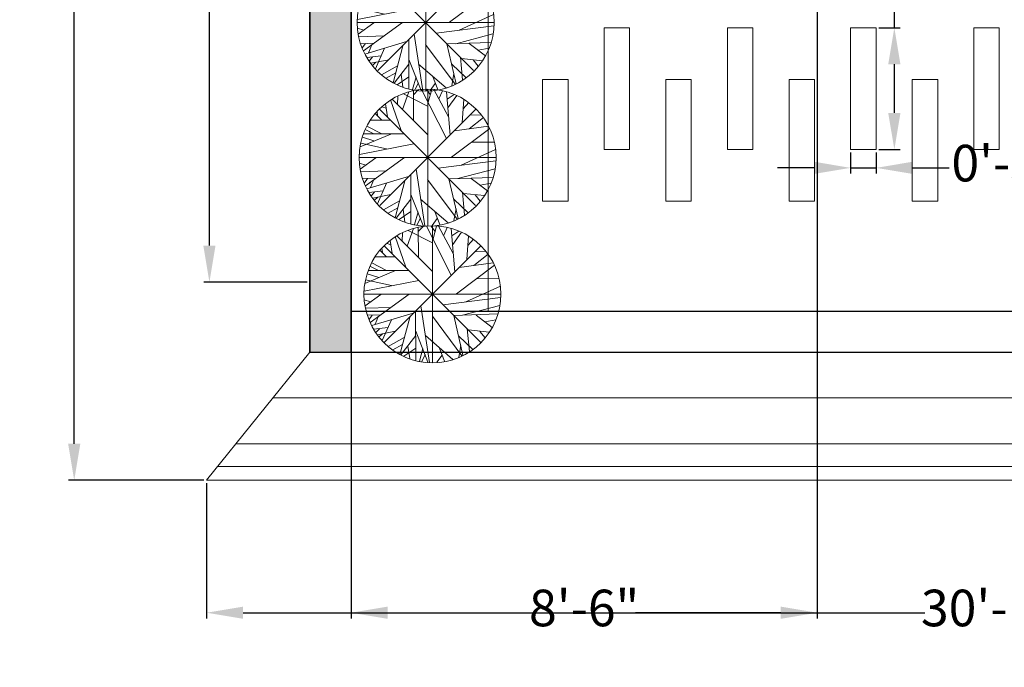
# Model space of a CAD drawing. Units: inches. Extents: x 2408 to 5087, y 2429 to 5085.
# Tile 1 of 12: x 2421 to 2636, y 2429 to 2570. Entities that reach past the tile are written whole.
import ezdxf

# ---------------------------------------------------------------- set-up
doc = ezdxf.new("R2010")
doc.units = ezdxf.units.IN
for name, color, linetype, lineweight in [('A-ANNO-DIMS', 2, 'Continuous', 18), ('A-FLOR', 7, 'Continuous', 25), ('A-FLOR-STRS', 7, 'Continuous', 18), ('A-WALL', 7, 'Continuous', 35), ('A-WALL-PATT', 252, 'Continuous', 13), ('L-HRDS-PVMT', 8, 'Continuous', 18), ('L-PLNT', 3, 'Continuous', 13)]:
    doc.layers.add(name, color=color, linetype=linetype, lineweight=lineweight)
doc.styles.get("Standard").update_dxf_attribs({"font": 'arial.ttf'})
doc.dimstyles.new('ISO-25', dxfattribs={"dimtxt": 8, "dimasz": 8, "dimexe": 1.25, "dimexo": 0.625, "dimtad": 0, "dimdec": 1, "dimlunit": 4, "dimtxsty": 'Standard', "dimcen": 2.5, "dimadec": 0, "dimazin": 0, "dimtfac": 1, "dimtdec": 1, "dimtmove": 0, "dimatfit": 3, "dimfxl": 1, "dimarcsym": 0})

# ---------------------------------------------------------------- blocks, each defined once
blk = doc.blocks.new('*D2')
at = {"layer": 'A-ANNO-DIMS', "color": 0, "lineweight": -2, "transparency": 16777216}
for p, q in [((2483.87, 3017.05), (2461.26, 3017.05)), ((2462.51, 3009.05), (2462.51, 2772.63)), ((2462.51, 2521.05), (2462.51, 2757.48)), ((2483.87, 2513.05), (2461.26, 2513.05))]:
    blk.add_line(p, q, dxfattribs=at)
at = {"layer": 'A-ANNO-DIMS', "color": 0, "transparency": 16777216}
for points in [[(2461.17, 3009.05), (2463.84, 3009.05), (2462.51, 3017.05)], [(2461.17, 2521.05), (2463.84, 2521.05), (2462.51, 2513.05)]]:
    blk.add_solid(points, dxfattribs=at)
at = {"layer": 'Defpoints', "color": 0, "transparency": 16777216}
for p in [(2484.49, 3017.05), (2462.51, 2513.05), (2484.49, 2513.05)]:
    blk.add_point(p, dxfattribs=at)
at = {"layer": 'A-ANNO-DIMS', "color": 0, "transparency": 16777216, "insert": (2462.51, 2765.05), "char_height": 8, "attachment_point": 5, "rotation": 90}
blk.add_mtext("42'", dxfattribs=at)
blk = doc.blocks.new('t2')
for p, q in [((3196.63, 2726.51), (3196.81, 2733.73)), ((3201.03, 2722), (3206.49, 2737.57)), ((3201.91, 2735.77), (3223.04, 2724.93)), ((3210.54, 2734.86), (3215.12, 2739.38)), ((3210.72, 2712.07), (3210.54, 2738.7)), ((3217.76, 2739.6), (3239.59, 2696.72)), ((3225.5, 2734.86), (3221.63, 2739.83)), ((3223.08, 2739.92), (3223.08, 2619.92)), ((3223.57, 2728.54), (3226.74, 2739.6)), ((3241.35, 2715.45), (3228.5, 2739.6)), ((3232.9, 2731.48), (3235.89, 2738.47)), ((3242.76, 2699.43), (3239.41, 2737.57)), ((3240.12, 2731.03), (3246.28, 2735.09)), ((3240.82, 2723.58), (3248.57, 2734.19)), ((3186.07, 2726.96), (3187.83, 2715.45)), ((3190.47, 2730.35), (3199.8, 2703.49)), ((3191.88, 2731.03), (3222.86, 2700.1)), ((3254.73, 2730.8), (3253.32, 2710.49)), ((3254.2, 2722.45), (3258.96, 2728.09)), ((3177.27, 2718.16), (3182.55, 2712.97)), ((3179.2, 2716.35), (3178.67, 2720.19)), ((3265.08, 2721.92), (3181.08, 2637.92)), ((3265.08, 2637.92), (3181.08, 2721.92)), ((3182.9, 2724.48), (3186.6, 2723.13)), ((3260.19, 2717.03), (3269.69, 2717.48)), ((3173.22, 2712.74), (3190.29, 2712.74)), ((3259.31, 2705.07), (3271.98, 2715)), ((3190.82, 2700.56), (3163.88, 2689.27)), ((3167.05, 2700.78), (3202.27, 2700.78)), ((3168.29, 2704.39), (3175.33, 2701.01)), ((3169.87, 2707.33), (3182.9, 2700.78)), ((3277.44, 2705.3), (3243.99, 2680.24)), ((3246.46, 2703.26), (3276.38, 2707.33)), ((3163.36, 2682.72), (3211.07, 2691.98)), ((3164.41, 2692.66), (3187.12, 2687.46)), ((3166, 2697.85), (3176.03, 2694.69)), ((3261.6, 2693.33), (3281.31, 2693.56)), ((3252.44, 2673.25), (3282.55, 2687.01)), ((3163.08, 2679.92), (3283.08, 2679.92)), ((3163.36, 2675.05), (3168.81, 2673.25)), ((3177.79, 2679.79), (3164.06, 2669.86)), ((3168.46, 2655.19), (3202.79, 2680.02)), ((3232.37, 2670.76), (3282.72, 2677.08)), ((3164.59, 2667.6), (3186.6, 2668.28)), ((3208.25, 2664.89), (3208.43, 2622.24)), ((3213, 2669.86), (3220.57, 2620.2)), ((3249.45, 2661.51), (3282.02, 2670.09)), ((3166, 2661.51), (3177.79, 2661.96)), ((3170.4, 2661.73), (3167.58, 2657.9)), ((3169.87, 2652.48), (3206.31, 2663.31)), ((3175.86, 2660.61), (3172.86, 2653.61)), ((3187.12, 2657.45), (3179.03, 2639.39)), ((3203.15, 2659.7), (3194.52, 2627.2)), ((3223.04, 2660.83), (3248.92, 2626.07)), ((3241.7, 2661.28), (3249.8, 2626.52)), ((3241.88, 2661.28), (3280.43, 2662.64)), ((3261.24, 2661.73), (3275.5, 2650.9)), ((3268.99, 2655.87), (3278.67, 2657.67)), ((3184.13, 2650.9), (3171.63, 2649.32)), ((3176.56, 2649.77), (3173.57, 2646.39)), ((3190.65, 2647.51), (3174.98, 2644.35)), ((3208.43, 2647.74), (3219.17, 2620.43)), ((3253.5, 2649.77), (3255.43, 2629.91)), ((3254.55, 2648.64), (3272.69, 2646.61)), ((3179.38, 2645.26), (3176.38, 2642.55)), ((3198.39, 2642.1), (3184.31, 2634.2)), ((3208.43, 2643.68), (3195.4, 2626.98)), ((3216.88, 2643.68), (3241, 2622.91)), ((3245.93, 2643.45), (3258.43, 2631.49)), ((3264.59, 2647.29), (3269.17, 2641.87)), ((3196.81, 2636), (3188.36, 2631.26)), ((3208.43, 2632.62), (3198.04, 2625.62)), ((3201.56, 2634.42), (3203.15, 2623.82)), ((3214.59, 2632.39), (3211.6, 2621.33)), ((3229.03, 2633.3), (3233.6, 2621.33)), ((3247.86, 2635.1), (3246.1, 2624.94)), ((3216.7, 2627.2), (3213.71, 2621.11)), ((3231.49, 2626.75), (3226.91, 2620.43))]:
    blk.add_line(p, q)
blk.add_circle((3223.08, 2679.92), 60)
blk = doc.blocks.new('PORTICO-PAVER')
blk.add_lwpolyline([(0, 26.64), (5.57, 26.64), (5.57, 0), (0, 0)], close=True)
blk = doc.blocks.new('*D27')
at = {"layer": 'A-ANNO-DIMS', "color": 0, "lineweight": -2, "transparency": 16777216}
for p, q in [((2612.36, 2568.68), (2612.36, 2576.68)), ((2608.98, 2568.68), (2613.61, 2568.68)), ((2612.36, 2550.04), (2612.36, 2560.68)), ((2608.98, 2542.04), (2613.61, 2542.04))]:
    blk.add_line(p, q, dxfattribs=at)
at = {"layer": 'A-ANNO-DIMS', "color": 0, "transparency": 16777216}
for points in [[(2611.02, 2560.68), (2613.69, 2560.68), (2612.36, 2568.68)], [(2611.02, 2550.04), (2613.69, 2550.04), (2612.36, 2542.04)]]:
    blk.add_solid(points, dxfattribs=at)
at = {"layer": 'Defpoints', "color": 0, "transparency": 16777216}
for p in [(2608.36, 2568.68), (2612.36, 2568.68), (2608.36, 2542.04)]:
    blk.add_point(p, dxfattribs=at)
at = {"layer": 'A-ANNO-DIMS', "color": 0, "transparency": 16777216, "insert": (2612.36, 2631.3), "char_height": 8, "attachment_point": 5, "rotation": 90}
blk.add_mtext('PAVER 2\'-2 1/2" TYP.', dxfattribs=at)
blk = doc.blocks.new('*D28')
at = {"layer": 'A-ANNO-DIMS', "color": 0, "lineweight": -2, "transparency": 16777216}
for p, q in [((2602.79, 2541.41), (2602.79, 2536.79)), ((2608.36, 2541.41), (2608.36, 2536.79)), ((2594.79, 2538.04), (2586.79, 2538.04)), ((2602.79, 2538.04), (2608.36, 2538.04)), ((2616.36, 2538.04), (2624.36, 2538.04))]:
    blk.add_line(p, q, dxfattribs=at)
at = {"layer": 'A-ANNO-DIMS', "color": 0, "transparency": 16777216}
for points in [[(2594.79, 2539.38), (2594.79, 2536.71), (2602.79, 2538.04)], [(2616.36, 2539.38), (2616.36, 2536.71), (2608.36, 2538.04)]]:
    blk.add_solid(points, dxfattribs=at)
at = {"layer": 'Defpoints', "color": 0, "transparency": 16777216}
for p in [(2602.79, 2542.04), (2608.36, 2542.04), (2608.36, 2538.04)]:
    blk.add_point(p, dxfattribs=at)
at = {"layer": 'A-ANNO-DIMS', "color": 0, "transparency": 16777216, "insert": (2658.69, 2538.04), "char_height": 8, "attachment_point": 5}
blk.add_mtext('0\'-5 1/2" TYP.', dxfattribs=at)
blk = doc.blocks.new('*D61')
at = {"layer": 'A-ANNO-DIMS', "color": 0, "lineweight": -2, "transparency": 16777216}
for p, q in [((2493.49, 2813.93), (2493.49, 2439.55)), ((2595.49, 2813.93), (2595.49, 2439.55)), ((2501.49, 2440.8), (2533.23, 2440.8)), ((2587.49, 2440.8), (2555.76, 2440.8))]:
    blk.add_line(p, q, dxfattribs=at)
at = {"layer": 'A-ANNO-DIMS', "color": 0, "transparency": 16777216}
for points in [[(2501.49, 2442.13), (2501.49, 2439.47), (2493.49, 2440.8)], [(2587.49, 2442.13), (2587.49, 2439.47), (2595.49, 2440.8)]]:
    blk.add_solid(points, dxfattribs=at)
at = {"layer": 'Defpoints', "color": 0, "transparency": 16777216}
for p in [(2493.49, 2814.55), (2595.49, 2814.55), (2595.49, 2440.8)]:
    blk.add_point(p, dxfattribs=at)
at = {"layer": 'A-ANNO-DIMS', "color": 0, "transparency": 16777216, "insert": (2544.49, 2440.8), "char_height": 8, "attachment_point": 5}
blk.add_mtext('8\'-6"', dxfattribs=at)
blk = doc.blocks.new('*D65')
at = {"layer": 'A-ANNO-DIMS', "color": 0, "lineweight": -2, "transparency": 16777216}
for p, q in [((2823.49, 2512.43), (2823.49, 2439.55)), ((2461.88, 2469.13), (2461.88, 2439.55)), ((2469.88, 2440.8), (2619, 2440.8)), ((2815.49, 2440.8), (2666.37, 2440.8))]:
    blk.add_line(p, q, dxfattribs=at)
at = {"layer": 'A-ANNO-DIMS', "color": 0, "transparency": 16777216}
for points in [[(2469.88, 2442.13), (2469.88, 2439.47), (2461.88, 2440.8)], [(2815.49, 2442.13), (2815.49, 2439.47), (2823.49, 2440.8)]]:
    blk.add_solid(points, dxfattribs=at)
at = {"layer": 'Defpoints', "color": 0, "transparency": 16777216}
for p in [(2823.49, 2513.05), (2461.88, 2469.75), (2823.49, 2440.8)]:
    blk.add_point(p, dxfattribs=at)
at = {"layer": 'A-ANNO-DIMS', "color": 0, "transparency": 16777216, "insert": (2642.69, 2440.8), "char_height": 8, "attachment_point": 5}
blk.add_mtext('30\'-1 1/2"', dxfattribs=at)
blk = doc.blocks.new('*D66')
at = {"layer": 'A-ANNO-DIMS', "color": 0, "lineweight": -2, "transparency": 16777216}
for p, q in [((2483.87, 3017.05), (2431.68, 3017.05)), ((2432.93, 3009.05), (2432.93, 2767.25)), ((2432.93, 2477.75), (2432.93, 2719.56)), ((2461.25, 2469.75), (2431.68, 2469.75))]:
    blk.add_line(p, q, dxfattribs=at)
at = {"layer": 'A-ANNO-DIMS', "color": 0, "transparency": 16777216}
for points in [[(2431.59, 3009.05), (2434.26, 3009.05), (2432.93, 3017.05)], [(2431.59, 2477.75), (2434.26, 2477.75), (2432.93, 2469.75)]]:
    blk.add_solid(points, dxfattribs=at)
at = {"layer": 'Defpoints', "color": 0, "transparency": 16777216}
for p in [(2432.93, 3017.05), (2484.49, 3017.05), (2461.88, 2469.75)]:
    blk.add_point(p, dxfattribs=at)
at = {"layer": 'A-ANNO-DIMS', "color": 0, "transparency": 16777216, "insert": (2432.93, 2743.4), "char_height": 8, "attachment_point": 5, "rotation": 90}
blk.add_mtext('45\'-7 1/2"', dxfattribs=at)

msp = doc.modelspace()

# ---------------------------------------------------------------- hatches: boundary and pattern name
at = {"layer": 'A-WALL-PATT'}
h = msp.add_hatch(color=256, dxfattribs=at)
h.dxf.hatch_style = 1
h.paths.add_polyline_path([(2493.49, 2613.55), (2523.49, 2613.55), (2523.49, 2622.55), (2493.49, 2622.55), (2493.49, 2714.8), (2484.49, 2714.8), (2484.49, 2497.75), (2493.49, 2497.75)])
h.paths.add_polyline_path([(2613.49, 2615.42), (2613.49, 2622.55), (2583.49, 2622.55), (2583.49, 2613.55), (2613.46, 2613.55, -0.009707)])
h.paths.add_polyline_path([(2823.49, 2634.55), (2814.49, 2634.55), (2814.49, 2622.55), (2694.49, 2622.55), (2694.49, 2670.55), (2706.49, 2670.55), (2706.49, 2675.05), (2694.49, 2675.05), (2694.49, 2750.05), (2685.49, 2750.05), (2685.49, 2622.55), (2661.49, 2622.55), (2661.49, 2613.55), (2814.49, 2613.55), (2814.49, 2522.05), (2688.49, 2522.05), (2688.49, 2513.05), (2823.49, 2513.05)])
h.paths.add_polyline_path([(2823.49, 2837.05), (2814.49, 2837.05), (2814.49, 2819.05), (2685.49, 2819.05), (2685.49, 2786.05), (2694.49, 2786.05), (2694.49, 2810.05), (2814.49, 2810.05), (2814.49, 2772.55), (2823.49, 2772.55)])
h.paths.add_polyline_path([(2694.49, 2964.55), (2595.49, 2964.55), (2595.49, 3008.05), (2601.49, 3008.05), (2601.49, 3017.05), (2484.49, 3017.05), (2484.49, 2972.05), (2493.49, 2972.05), (2493.49, 3008.05), (2586.49, 3008.05), (2586.49, 2955.55), (2685.49, 2955.55), (2685.49, 2854.87), (2694.49, 2854.87)])
h.paths.add_polyline_path([(2493.49, 2867.05), (2595.49, 2867.05), (2595.49, 2876.05), (2493.49, 2876.05), (2493.49, 2912.05), (2484.49, 2912.05), (2484.49, 2774.8), (2493.49, 2774.8)])
h.paths.add_polyline_path([(2595.49, 2814.55), (2493.49, 2814.55), (2493.49, 2810.05), (2595.49, 2810.05)], flags=17)
h.paths.add_polyline_path([(2724.49, 3017.05), (2625.49, 3017.05), (2625.49, 3008.05), (2685.49, 3008.05), (2685.49, 2994.55), (2694.49, 2994.55), (2694.49, 3008.05), (2724.49, 3008.05)])
h.paths.add_polyline_path([(2823.49, 3017.05), (2784.49, 3017.05), (2784.49, 3008.05), (2814.49, 3008.05), (2814.49, 2913.55), (2814.56, 2897.05), (2823.49, 2897.05)])
h.paths.add_polyline_path([(2823.49, 2712.55), (2814.61, 2712.55), (2814.66, 2701.27), (2814.49, 2701.27), (2814.49, 2675.05), (2740.99, 2675.05), (2740.99, 2687.05), (2736.49, 2687.05), (2736.49, 2670.55), (2814.49, 2670.55), (2814.49, 2658.55), (2823.49, 2658.55)], flags=17)

# ---------------------------------------------------------------- linework, layer by layer
at = {"layer": 'A-FLOR'}
for p, q in [((2493.49, 2506.75), (2688.49, 2506.75)), ((2484.49, 2497.75), (2688.49, 2497.75))]:
    msp.add_line(p, q, dxfattribs=at)
at = {"layer": 'A-FLOR-STRS'}
for p, q in [((2484.49, 2497.75), (2461.88, 2469.75)), ((2476.42, 2487.75), (2688.49, 2487.75)), ((2468.34, 2477.75), (2698.49, 2477.75)), ((2464.3, 2472.75), (2708.49, 2472.75)), ((2461.88, 2469.75), (2708.49, 2469.75))]:
    msp.add_line(p, q, dxfattribs=at)
at = {"layer": 'A-WALL'}
for p, q in [((2484.49, 3017.05), (2484.49, 2497.75)), ((2493.49, 2613.55), (2493.49, 2497.75))]:
    msp.add_line(p, q, dxfattribs=at)
at = {"layer": 'L-PLNT'}
msp.add_line((2523.49, 2613.55), (2523.49, 2506.75), dxfattribs=at)

# ---------------------------------------------------------------- block references
at = {"layer": 'L-HRDS-PVMT'}
for p in [(2548.88, 2542.04), (2575.83, 2542.04), (2602.79, 2542.04), (2629.74, 2542.04), (2535.4, 2530.73), (2562.36, 2530.73), (2589.31, 2530.73), (2616.27, 2530.73)]:
    msp.add_blockref('PORTICO-PAVER', p, dxfattribs=at)
at = {"layer": 'L-PLNT', "xscale": 0.2497966910751513, "yscale": 0.2497966910751513, "zscale": 0.2497966910751513}
for p in [(1704.71, 1900.35), (1705.15, 1870.85), (1706.19, 1840.98)]:
    msp.add_blockref('t2', p, dxfattribs=at)

# ---------------------------------------------------------------- dimensions: what is measured, and where the dimension line sits
at = {"layer": 'A-ANNO-DIMS'}
for base, p1, p2, override, picture, middle in [((2432.93, 3017.05), (2461.88, 2469.75), (2484.49, 3017.05), {"dimdec": 1, "dimlfac": 1, "dimrnd": 0, "dimzin": 1, "dimdsep": 46, "dimlunit": 4, "dimfrac": 2}, '*D66', (2432.93, 2743.4)), ((2462.51, 2513.05), (2484.49, 3017.05), (2484.49, 2513.05), {"dimclrd": 0, "dimclre": 0, "dimclrt": 0}, '*D2', (2462.51, 2765.05))]:
    dim = msp.add_linear_dim(base=base, p1=p1, p2=p2, angle=90, dimstyle='ISO-25', override=override, dxfattribs=at)
    dim.commit()
    dim.dimension.update_dxf_attribs({"geometry": picture, "text_midpoint": middle})
for base, p1, p2, picture, middle in [((2595.49, 2440.8), (2493.49, 2814.55), (2595.49, 2814.55), '*D61', (2544.49, 2440.8)), ((2823.49, 2440.8), (2461.88, 2469.75), (2823.49, 2513.05), '*D65', (2642.69, 2440.8))]:
    dim = msp.add_linear_dim(base=base, p1=p1, p2=p2, dimstyle='ISO-25', override={"dimdec": 1, "dimlfac": 1, "dimrnd": 0, "dimzin": 1, "dimdsep": 46, "dimlunit": 4, "dimfrac": 2}, dxfattribs=at)
    dim.commit()
    dim.dimension.update_dxf_attribs({"geometry": picture, "text_midpoint": middle})
dim = msp.add_linear_dim(base=(2612.36, 2568.68), p1=(2608.36, 2542.04), p2=(2608.36, 2568.68), angle=90, text='PAVER <> TYP.', dimstyle='ISO-25', override={"dimdec": 1, "dimlfac": 1, "dimrnd": 0, "dimzin": 1, "dimdsep": 46, "dimlunit": 4, "dimfrac": 2}, dxfattribs=at)
dim.commit()
dim.dimension.update_dxf_attribs({"geometry": '*D27', "text_midpoint": (2612.36, 2631.3)})
dim = msp.add_linear_dim(base=(2608.36, 2538.04), p1=(2602.79, 2542.04), p2=(2608.36, 2542.04), text='<> TYP.', dimstyle='ISO-25', override={"dimdec": 1, "dimlfac": 1, "dimrnd": 0, "dimzin": 1, "dimdsep": 46, "dimlunit": 4, "dimfrac": 2}, dxfattribs=at)
dim.commit()
dim.dimension.update_dxf_attribs({"geometry": '*D28', "text_midpoint": (2658.69, 2538.04)})

doc.saveas('drawing.dxf')
